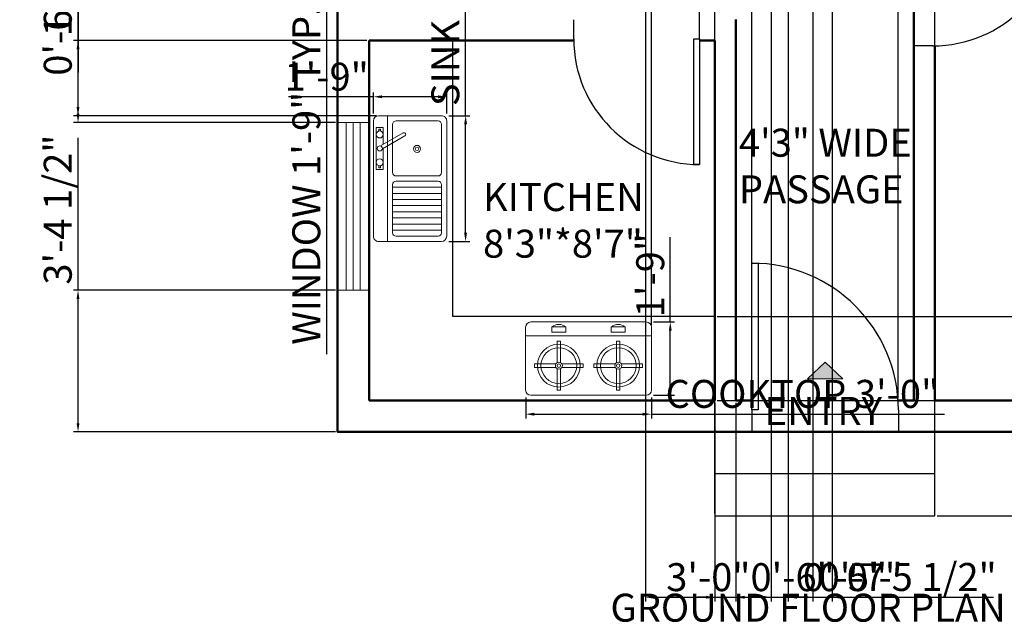
# Model space of a CAD drawing. Units: inches. Extents: x 2528 to 2954, y 1660 to 2209.
# Tile 1 of 4: x 2528 to 2810, y 1660 to 1832. Entities that reach past the tile are written whole.
import ezdxf

# ---------------------------------------------------------------- set-up
doc = ezdxf.new("R2010")
doc.units = ezdxf.units.IN
for name, color, linetype, lineweight in [('A-ANNO-DIMS', 5, 'Continuous', 18), ('A-ANNO-SYMB', 5, 'Continuous', 18), ('A-AREA-IDEN', 5, 'Continuous', 25), ('A-EQPM', 6, 'Continuous', 18), ('A-FLOR-CASE', 32, 'Continuous', 25), ('A-FLOR-FIXT', 6, 'Continuous', 18), ('DOOR', 3, 'Continuous', 25), ('STEPS', 30, 'Continuous', 25), ('TEXT', 5, 'Continuous', 25), ('WALL', 1, 'Continuous', 50), ('WINDOW', 4, 'Continuous', 18)]:
    doc.layers.add(name, color=color, linetype=linetype, lineweight=lineweight)
doc.styles.get("Standard").update_dxf_attribs({"font": 'arial.ttf'})
doc.dimstyles.new('ISO-25', dxfattribs={"dimtxt": 8, "dimasz": 2.5, "dimexe": 1.25, "dimexo": 0.625, "dimtad": 1, "dimlunit": 3, "dimtxsty": 'Standard', "dimcen": 2.5, "dimadec": 0, "dimazin": 0, "dimtfac": 1, "dimtmove": 0, "dimatfit": 3, "dimfxl": 1, "dimarcsym": 0})

# ---------------------------------------------------------------- blocks, each defined once
blk = doc.blocks.new('*U2')
for p, q in [((0, 0), (0, -6)), ((40, 0), (40, -6))]:
    blk.add_line(p, q)
blk.add_lwpolyline([(0, 0), (0, 40), (1.75, 40), (1.75, 0)], close=True)
blk.add_arc((0, 0), 40, 0, 90)
blk = doc.blocks.new('Faucet - kit sink top')
for p, q in [((-5.5, -0.75), (-5.5, -1.25)), ((-4.94278, -0.75), (-5.5, -0.75)), ((-5.5, -1.25), (-4.94278, -1.25)), ((-0.14775, -1.7441), (3.56698, -8.1782)), ((4.43301, -7.6782), (0.71828, -1.2441)), ((4.94278, -0.75), (5.5, -0.75)), ((5.5, -1.25), (4.94278, -1.25)), ((5.5, -0.75), (5.5, -1.25))]:
    blk.add_line(p, q)
blk.add_lwpolyline([(-0.00587, -2), (-6, -2), (-6, 0), (6, 0), (6, -2), (1.15195, -2)])
for centre, radius in [((-4, -1), 1), ((4, -1), 1), ((0, -1), 0.75)]:
    blk.add_circle(centre, radius)
blk.add_arc((4, -7.9282), 0.5, 210, 30)
blk = doc.blocks.new('sink')
for p, q in [((-18, -4), (18, -4)), ((-14.75, -19.5), (-14.75, -5.5)), ((-13, -19.5), (-13, -5.5)), ((-11.25, -19.5), (-11.25, -5.5)), ((-9.5, -19.5), (-9.5, -5.5)), ((-7.75, -19.5), (-7.75, -5.5)), ((-6, -19.5), (-6, -5.5)), ((-4.25, -19.5), (-4.25, -5.5)), ((-2.5, -19.5), (-2.5, -5.5)), ((-0.75, -18.5), (-0.75, -6.5)), ((0.75, -6.5), (0.75, -18.5))]:
    blk.add_line(p, q)
for points in [[(-16.5, 0), (16.5, 0)], [(-18, -19.5), (-18, -1.5)], [(18, -1.5), (18, -19.5)], [(-15.5, -5.5), (-1.75, -5.5)], [(1.75, -5.5), (15.5, -5.5)], [(-16.5, -18.5), (-16.5, -6.5)], [(16.5, -6.5), (16.5, -18.5)], [(-1.75, -19.5), (-15.5, -19.5)], [(15.5, -19.5), (1.75, -19.5)], [(16.5, -21), (-16.5, -21)]]:
    blk.add_lwpolyline(points)
for radius in [1, 0.5]:
    blk.add_circle((8.5, -12.5), radius)
for centre, radius, start, end in [((-16.5, -1.5), 1.5, 90, 180), ((16.5, -1.5), 1.5, 0, 90), ((-15.5, -6.5), 1, 90, 180), ((-1.75, -6.5), 1, 0, 90), ((1.75, -6.5), 1, 90, 180), ((15.5, -6.5), 1, 0, 90), ((-16.5, -19.5), 1.5, 180, 270), ((-15.5, -18.5), 1, 180, 270), ((-1.75, -18.5), 1, 270, 0), ((1.75, -18.5), 1, 180, 270), ((15.5, -18.5), 1, 270, 0), ((16.5, -19.5), 1.5, 270, 0)]:
    blk.add_arc(centre, radius, start, end)
blk.add_blockref('Faucet - kit sink top', (8.62, -0.83))
blk = doc.blocks.new('stove')
for p, q in [((2468.66, 1798.42), (2464.66, 1798.42)), ((2464.66, 1798.42), (2464.66, 1796.93)), ((2468.66, 1796.93), (2468.66, 1798.42)), ((2485.66, 1798.42), (2481.66, 1798.42)), ((2481.66, 1798.42), (2481.66, 1796.93)), ((2485.66, 1796.93), (2485.66, 1798.42)), ((2457.16, 1795.87), (2493.16, 1795.87)), ((2464.66, 1796.93), (2468.66, 1796.93)), ((2481.66, 1796.93), (2485.66, 1796.93))]:
    blk.add_line(p, q)
for points in [[(2457.16, 1780.37), (2457.16, 1798.37)], [(2458.66, 1799.87), (2491.66, 1799.87)], [(2493.16, 1798.37), (2493.16, 1780.37)], [(2491.66, 1778.87), (2458.66, 1778.87)]]:
    blk.add_lwpolyline(points)
for centre, radius in [((2466.66, 1787.37), 6.12), ((2483.66, 1787.37), 6.12), ((2466.66, 1787.37), 5.12), ((2483.66, 1787.37), 5.12), ((2466.66, 1787.37), 1), ((2466.66, 1787.37), 0.5), ((2483.66, 1787.37), 1), ((2483.66, 1787.37), 0.5)]:
    blk.add_circle(centre, radius)
for centre, radius, start, end in [((2458.66, 1798.37), 1.5, 90, 180), ((2466.66, 1796.04), 3.11, 49.9196, 130.0804), ((2483.66, 1796.04), 3.11, 49.9196, 130.0804), ((2491.66, 1798.37), 1.5, 0, 90), ((2458.66, 1780.37), 1.5, 180, 270), ((2491.66, 1780.37), 1.5, 270, 0)]:
    blk.add_arc(centre, radius, start, end)
blk = doc.blocks.new('stove kitchen')
for p, q in [((-9, 9.37), (-9, 15.48)), ((-9, 15.48), (-8, 15.48)), ((-8, 9.37), (-8, 15.48)), ((8, 9.37), (8, 15.48)), ((8, 15.48), (9, 15.48)), ((9, 9.37), (9, 15.48)), ((-9.37, 9), (-15.48, 9)), ((-15.48, 9), (-15.48, 8)), ((-7.63, 9), (-1.52, 9)), ((-1.52, 8), (-1.52, 9)), ((7.63, 9), (1.52, 9)), ((1.52, 9), (1.52, 8)), ((9.37, 9), (15.48, 9)), ((15.48, 8), (15.48, 9)), ((-9.37, 8), (-15.48, 8)), ((-9, 7.63), (-9, 1.52)), ((-8, 7.63), (-8, 1.52)), ((-7.63, 8), (-1.52, 8)), ((7.63, 8), (1.52, 8)), ((8, 7.63), (8, 1.52)), ((9, 7.63), (9, 1.52)), ((9.37, 8), (15.48, 8)), ((-8, 1.52), (-9, 1.52)), ((9, 1.52), (8, 1.52))]:
    blk.add_line(p, q)
blk.add_blockref('stove', (-2475.16, -1778.87))
blk = doc.blocks.new('WIN-48IN')
for p, q in [((0, 48), (9, 48)), ((2.5, 0), (2.5, 48)), ((4.5, 0), (4.5, 48)), ((6.5, 0), (6.5, 48)), ((9, 0), (0, 0))]:
    blk.add_line(p, q)
blk = doc.blocks.new('*D19')
at = {"layer": 'A-ANNO-DIMS', "color": 0, "lineweight": -2, "transparency": 16777216}
for p, q in [((2618.29, 1862.65), (2614.52, 1862.65)), ((2615.77, 1860.15), (2615.77, 1844.15)), ((2618.29, 1841.65), (2614.52, 1841.65)), ((2615.77, 1841.65), (2615.77, 1736.66))]:
    blk.add_line(p, q, dxfattribs=at)
at = {"layer": 'A-ANNO-DIMS', "color": 0, "transparency": 16777216}
for points in [[(2615.35, 1860.15), (2616.18, 1860.15), (2615.77, 1862.65)], [(2615.35, 1844.15), (2616.18, 1844.15), (2615.77, 1841.65)]]:
    blk.add_solid(points, dxfattribs=at)
at = {"layer": 'Defpoints', "color": 0, "transparency": 16777216}
for p in [(2618.92, 1862.65), (2615.77, 1841.65), (2618.92, 1841.65)]:
    blk.add_point(p, dxfattribs=at)
at = {"layer": 'A-ANNO-DIMS', "color": 0, "transparency": 16777216, "insert": (2611, 1787.9), "char_height": 8, "attachment_point": 5, "rotation": 90}
blk.add_mtext('WINDOW 1\'-9" TYP.', dxfattribs=at)
blk = doc.blocks.new('*D23')
at = {"layer": 'A-ANNO-DIMS', "color": 0, "lineweight": -2, "transparency": 16777216}
for p, q in [((2655.56, 1804.89), (2655.56, 1859.06)), ((2650.79, 1804.89), (2656.81, 1804.89)), ((2655.56, 1771.39), (2655.56, 1802.39)), ((2650.79, 1768.89), (2656.81, 1768.89))]:
    blk.add_line(p, q, dxfattribs=at)
at = {"layer": 'A-ANNO-DIMS', "color": 0, "transparency": 16777216}
for points in [[(2655.15, 1802.39), (2655.98, 1802.39), (2655.56, 1804.89)], [(2655.15, 1771.39), (2655.98, 1771.39), (2655.56, 1768.89)]]:
    blk.add_solid(points, dxfattribs=at)
at = {"layer": 'Defpoints', "color": 0, "transparency": 16777216}
for p in [(2650.16, 1804.89), (2655.56, 1804.89), (2650.16, 1768.89)]:
    blk.add_point(p, dxfattribs=at)
at = {"layer": 'A-ANNO-DIMS', "color": 0, "transparency": 16777216, "insert": (2650.8, 1833.22), "char_height": 8, "attachment_point": 5, "rotation": 90}
blk.add_mtext('SINK 3\'-0"', dxfattribs=at)
blk = doc.blocks.new('*D24')
at = {"layer": 'A-ANNO-DIMS', "color": 0, "lineweight": -2, "transparency": 16777216}
for p, q in [((2629.16, 1810.29), (2604.9, 1810.29)), ((2629.16, 1805.51), (2629.16, 1811.54)), ((2647.66, 1810.29), (2631.66, 1810.29)), ((2650.16, 1805.51), (2650.16, 1811.54))]:
    blk.add_line(p, q, dxfattribs=at)
at = {"layer": 'A-ANNO-DIMS', "color": 0, "transparency": 16777216}
for points in [[(2631.66, 1810.71), (2631.66, 1809.87), (2629.16, 1810.29)], [(2647.66, 1810.71), (2647.66, 1809.87), (2650.16, 1810.29)]]:
    blk.add_solid(points, dxfattribs=at)
at = {"layer": 'Defpoints', "color": 0, "transparency": 16777216}
for p in [(2629.16, 1810.29), (2629.16, 1804.89), (2650.16, 1804.89)]:
    blk.add_point(p, dxfattribs=at)
at = {"layer": 'A-ANNO-DIMS', "color": 0, "transparency": 16777216, "insert": (2615.78, 1815), "char_height": 8, "attachment_point": 5}
blk.add_mtext('1\'-9"', dxfattribs=at)
blk = doc.blocks.new('*D25')
at = {"layer": 'A-ANNO-DIMS', "color": 0, "lineweight": -2, "transparency": 16777216}
for p, q in [((2672.76, 1724.24), (2672.76, 1718.22)), ((2708.76, 1724.24), (2708.76, 1718.22)), ((2675.26, 1719.47), (2706.26, 1719.47)), ((2708.76, 1719.47), (2792.67, 1719.47))]:
    blk.add_line(p, q, dxfattribs=at)
at = {"layer": 'A-ANNO-DIMS', "color": 0, "transparency": 16777216}
for points in [[(2675.26, 1719.89), (2675.26, 1719.05), (2672.76, 1719.47)], [(2706.26, 1719.89), (2706.26, 1719.05), (2708.76, 1719.47)]]:
    blk.add_solid(points, dxfattribs=at)
at = {"layer": 'Defpoints', "color": 0, "transparency": 16777216}
for p in [(2672.76, 1724.87), (2708.76, 1724.87), (2708.76, 1719.47)]:
    blk.add_point(p, dxfattribs=at)
at = {"layer": 'A-ANNO-DIMS', "color": 0, "transparency": 16777216, "insert": (2751.96, 1724.24), "char_height": 8, "attachment_point": 5}
blk.add_mtext('COOKTOP 3\'-0"', dxfattribs=at)
blk = doc.blocks.new('*D26')
at = {"layer": 'A-ANNO-DIMS', "color": 0, "lineweight": -2, "transparency": 16777216}
for p, q in [((2714.16, 1745.87), (2714.16, 1770.13)), ((2709.38, 1745.87), (2715.41, 1745.87)), ((2714.16, 1727.37), (2714.16, 1743.37)), ((2709.38, 1724.87), (2715.41, 1724.87))]:
    blk.add_line(p, q, dxfattribs=at)
at = {"layer": 'A-ANNO-DIMS', "color": 0, "transparency": 16777216}
for points in [[(2713.74, 1743.37), (2714.57, 1743.37), (2714.16, 1745.87)], [(2713.74, 1727.37), (2714.57, 1727.37), (2714.16, 1724.87)]]:
    blk.add_solid(points, dxfattribs=at)
at = {"layer": 'Defpoints', "color": 0, "transparency": 16777216}
for p in [(2708.76, 1745.87), (2714.16, 1745.87), (2708.76, 1724.87)]:
    blk.add_point(p, dxfattribs=at)
at = {"layer": 'A-ANNO-DIMS', "color": 0, "transparency": 16777216, "insert": (2709.45, 1759.25), "char_height": 8, "attachment_point": 5, "rotation": 90}
blk.add_mtext('1\'-9"', dxfattribs=at)
blk = doc.blocks.new('*D27')
at = {"layer": 'A-ANNO-DIMS', "color": 0, "lineweight": -2, "transparency": 16777216}
for p, q in [((2544.62, 1754.93), (2544.62, 1798.58)), ((2618.29, 1754.93), (2543.37, 1754.93)), ((2544.62, 1716.89), (2544.62, 1752.43)), ((2618.29, 1714.39), (2543.37, 1714.39))]:
    blk.add_line(p, q, dxfattribs=at)
at = {"layer": 'A-ANNO-DIMS', "color": 0, "transparency": 16777216}
for points in [[(2544.2, 1752.43), (2545.03, 1752.43), (2544.62, 1754.93)], [(2544.2, 1716.89), (2545.03, 1716.89), (2544.62, 1714.39)]]:
    blk.add_solid(points, dxfattribs=at)
at = {"layer": 'Defpoints', "color": 0, "transparency": 16777216}
for p in [(2544.62, 1754.93), (2618.92, 1754.93), (2618.92, 1714.39)]:
    blk.add_point(p, dxfattribs=at)
at = {"layer": 'A-ANNO-DIMS', "color": 0, "transparency": 16777216, "insert": (2539.85, 1778), "char_height": 8, "attachment_point": 5, "rotation": 90}
blk.add_mtext('3\'-4 1/2"', dxfattribs=at)
blk = doc.blocks.new('*D28')
at = {"layer": 'A-ANNO-DIMS', "color": 0, "lineweight": -2, "transparency": 16777216}
for p, q in [((2544.62, 1841.65), (2544.62, 1885.3)), ((2618.29, 1841.65), (2543.37, 1841.65)), ((2544.62, 1805.43), (2544.62, 1839.14)), ((2618.29, 1802.93), (2543.37, 1802.93))]:
    blk.add_line(p, q, dxfattribs=at)
at = {"layer": 'A-ANNO-DIMS', "color": 0, "transparency": 16777216}
for points in [[(2544.2, 1839.14), (2545.03, 1839.14), (2544.62, 1841.65)], [(2544.2, 1805.43), (2545.03, 1805.43), (2544.62, 1802.93)]]:
    blk.add_solid(points, dxfattribs=at)
at = {"layer": 'Defpoints', "color": 0, "transparency": 16777216}
for p in [(2544.62, 1841.65), (2618.92, 1841.65), (2618.92, 1802.93)]:
    blk.add_point(p, dxfattribs=at)
at = {"layer": 'A-ANNO-DIMS', "color": 0, "transparency": 16777216, "insert": (2539.85, 1864.72), "char_height": 8, "attachment_point": 5, "rotation": 90}
blk.add_mtext('3\'-2 1/2"', dxfattribs=at)
blk = doc.blocks.new('*D34')
at = {"layer": 'A-ANNO-DIMS', "color": 0, "lineweight": -2, "transparency": 16777216}
for p, q in [((2618.92, 1715.01), (2618.92, 2122.94)), ((2726.92, 1703.01), (2726.92, 2122.94)), ((2621.42, 2121.69), (2724.42, 2121.69))]:
    blk.add_line(p, q, dxfattribs=at)
at = {"layer": 'A-ANNO-DIMS', "color": 0, "transparency": 16777216}
for points in [[(2621.42, 2122.11), (2621.42, 2121.27), (2618.92, 2121.69)], [(2724.42, 2122.11), (2724.42, 2121.27), (2726.92, 2121.69)]]:
    blk.add_solid(points, dxfattribs=at)
at = {"layer": 'Defpoints', "color": 0, "transparency": 16777216}
for p in [(2726.92, 2121.69), (2618.92, 1714.39), (2726.92, 1702.39)]:
    blk.add_point(p, dxfattribs=at)
at = {"layer": 'A-ANNO-DIMS', "color": 0, "transparency": 16777216, "insert": (2672.92, 2126.4), "char_height": 8, "attachment_point": 5}
blk.add_mtext('9\'-0"', dxfattribs=at)
blk = doc.blocks.new('*D35')
at = {"layer": 'A-ANNO-DIMS', "color": 0, "lineweight": -2, "transparency": 16777216}
for p, q in [((2726.92, 1691.01), (2726.92, 2122.94)), ((2789.92, 1691.01), (2789.92, 2122.94)), ((2729.42, 2121.69), (2787.42, 2121.69))]:
    blk.add_line(p, q, dxfattribs=at)
at = {"layer": 'A-ANNO-DIMS', "color": 0, "transparency": 16777216}
for points in [[(2729.42, 2122.11), (2729.42, 2121.27), (2726.92, 2121.69)], [(2787.42, 2122.11), (2787.42, 2121.27), (2789.92, 2121.69)]]:
    blk.add_solid(points, dxfattribs=at)
at = {"layer": 'Defpoints', "color": 0, "transparency": 16777216}
for p in [(2789.92, 2121.69), (2726.92, 1690.39), (2789.92, 1690.39)]:
    blk.add_point(p, dxfattribs=at)
at = {"layer": 'A-ANNO-DIMS', "color": 0, "transparency": 16777216, "insert": (2758.42, 2126.4), "char_height": 8, "attachment_point": 5}
blk.add_mtext('5\'-3"', dxfattribs=at)
blk = doc.blocks.new('*D36')
at = {"layer": 'A-ANNO-DIMS', "color": 0, "lineweight": -2, "transparency": 16777216}
for p, q in [((2790.54, 1714.39), (2943.47, 1714.39)), ((2942.22, 1692.89), (2942.22, 1711.89)), ((2790.54, 1690.39), (2943.47, 1690.39))]:
    blk.add_line(p, q, dxfattribs=at)
at = {"layer": 'A-ANNO-DIMS', "color": 0, "transparency": 16777216}
for points in [[(2941.8, 1711.89), (2942.63, 1711.89), (2942.22, 1714.39)], [(2941.8, 1692.89), (2942.63, 1692.89), (2942.22, 1690.39)]]:
    blk.add_solid(points, dxfattribs=at)
at = {"layer": 'Defpoints', "color": 0, "transparency": 16777216}
for p in [(2789.92, 1714.39), (2942.22, 1714.39), (2789.92, 1690.39)]:
    blk.add_point(p, dxfattribs=at)
at = {"layer": 'A-ANNO-DIMS', "color": 0, "transparency": 16777216, "insert": (2937.51, 1702.39), "char_height": 8, "attachment_point": 5, "rotation": 90}
blk.add_mtext('2\'-0"', dxfattribs=at)
blk = doc.blocks.new('*D37')
at = {"layer": 'A-ANNO-DIMS', "color": 0, "lineweight": -2, "transparency": 16777216}
for p, q in [((2737.46, 1724.01), (2737.46, 2122.94)), ((2779.37, 1724.01), (2779.37, 2122.94)), ((2739.96, 2121.69), (2776.87, 2121.69))]:
    blk.add_line(p, q, dxfattribs=at)
at = {"layer": 'A-ANNO-DIMS', "color": 0, "transparency": 16777216}
for points in [[(2739.96, 2122.11), (2739.96, 2121.27), (2737.46, 2121.69)], [(2776.87, 2122.11), (2776.87, 2121.27), (2779.37, 2121.69)]]:
    blk.add_solid(points, dxfattribs=at)
at = {"layer": 'Defpoints', "color": 0, "transparency": 16777216}
for p in [(2779.37, 2121.69), (2737.46, 1723.39), (2779.37, 1723.39)]:
    blk.add_point(p, dxfattribs=at)
at = {"layer": 'A-ANNO-DIMS', "color": 0, "transparency": 16777216, "insert": (2758.42, 2126.4), "char_height": 8, "attachment_point": 5}
blk.add_mtext('3\'-6"', dxfattribs=at)
blk = doc.blocks.new('*D38')
at = {"layer": 'A-ANNO-DIMS', "color": 0, "lineweight": -2, "transparency": 16777216}
for p, q in [((2707.05, 1956.76), (2707.05, 1665.84)), ((2743.05, 1956.76), (2743.05, 1665.84)), ((2709.55, 1667.09), (2740.55, 1667.09))]:
    blk.add_line(p, q, dxfattribs=at)
at = {"layer": 'A-ANNO-DIMS', "color": 0, "transparency": 16777216}
for points in [[(2709.55, 1667.51), (2709.55, 1666.67), (2707.05, 1667.09)], [(2740.55, 1667.51), (2740.55, 1666.67), (2743.05, 1667.09)]]:
    blk.add_solid(points, dxfattribs=at)
at = {"layer": 'Defpoints', "color": 0, "transparency": 16777216}
for p in [(2707.05, 1957.39), (2743.05, 1957.39), (2743.05, 1667.09)]:
    blk.add_point(p, dxfattribs=at)
at = {"layer": 'A-ANNO-DIMS', "color": 0, "transparency": 16777216, "insert": (2725.05, 1671.8), "char_height": 8, "attachment_point": 5}
blk.add_mtext('3\'-0"', dxfattribs=at)
blk = doc.blocks.new('*D44')
at = {"layer": 'A-ANNO-DIMS', "color": 0, "lineweight": -2, "transparency": 16777216}
for p, q in [((2727.54, 1747.39), (2943.47, 1747.39)), ((2942.22, 1725.89), (2942.22, 1744.89)), ((2727.54, 1723.39), (2943.47, 1723.39))]:
    blk.add_line(p, q, dxfattribs=at)
at = {"layer": 'A-ANNO-DIMS', "color": 0, "transparency": 16777216}
for points in [[(2941.8, 1744.89), (2942.63, 1744.89), (2942.22, 1747.39)], [(2941.8, 1725.89), (2942.63, 1725.89), (2942.22, 1723.39)]]:
    blk.add_solid(points, dxfattribs=at)
at = {"layer": 'Defpoints', "color": 0, "transparency": 16777216}
for p in [(2726.92, 1747.39), (2942.22, 1747.39), (2726.92, 1723.39)]:
    blk.add_point(p, dxfattribs=at)
at = {"layer": 'A-ANNO-DIMS', "color": 0, "transparency": 16777216, "insert": (2937.51, 1735.39), "char_height": 8, "attachment_point": 5, "rotation": 90}
blk.add_mtext('2\'-0"', dxfattribs=at)
blk = doc.blocks.new('*D45')
at = {"layer": 'A-ANNO-DIMS', "color": 0, "lineweight": -2, "transparency": 16777216}
for p, q in [((2708.76, 1744.99), (2708.76, 2122.94)), ((2726.92, 1748.01), (2726.92, 2122.94)), ((2711.26, 2121.69), (2724.42, 2121.69)), ((2726.92, 2121.69), (2751.18, 2121.69))]:
    blk.add_line(p, q, dxfattribs=at)
at = {"layer": 'A-ANNO-DIMS', "color": 0, "transparency": 16777216}
for points in [[(2711.26, 2122.11), (2711.26, 2121.27), (2708.76, 2121.69)], [(2724.42, 2122.11), (2724.42, 2121.27), (2726.92, 2121.69)]]:
    blk.add_solid(points, dxfattribs=at)
at = {"layer": 'Defpoints', "color": 0, "transparency": 16777216}
for p in [(2726.92, 2121.69), (2726.92, 1747.39), (2708.76, 1744.37)]:
    blk.add_point(p, dxfattribs=at)
at = {"layer": 'A-ANNO-DIMS', "color": 0, "transparency": 16777216, "insert": (2740.3, 2126.4), "char_height": 8, "attachment_point": 5}
blk.add_mtext('1\'-6"', dxfattribs=at)
blk = doc.blocks.new('*D46')
at = {"layer": 'A-ANNO-DIMS', "color": 0, "lineweight": -2, "transparency": 16777216}
for p, q in [((2544.62, 1826.39), (2544.62, 1869.29)), ((2627.29, 1826.39), (2543.37, 1826.39)), ((2544.62, 1807.39), (2544.62, 1823.89)), ((2630.04, 1804.89), (2543.37, 1804.89))]:
    blk.add_line(p, q, dxfattribs=at)
at = {"layer": 'A-ANNO-DIMS', "color": 0, "transparency": 16777216}
for points in [[(2544.2, 1823.89), (2545.03, 1823.89), (2544.62, 1826.39)], [(2544.2, 1807.39), (2545.03, 1807.39), (2544.62, 1804.89)]]:
    blk.add_solid(points, dxfattribs=at)
at = {"layer": 'Defpoints', "color": 0, "transparency": 16777216}
for p in [(2544.62, 1826.39), (2627.92, 1826.39), (2630.66, 1804.89)]:
    blk.add_point(p, dxfattribs=at)
at = {"layer": 'A-ANNO-DIMS', "color": 0, "transparency": 16777216, "insert": (2539.85, 1849.09), "char_height": 8, "attachment_point": 5, "rotation": 90}
blk.add_mtext('1\'-9 1/2"', dxfattribs=at)
blk = doc.blocks.new('*D48')
at = {"layer": 'A-ANNO-DIMS', "color": 0, "lineweight": -2, "transparency": 16777216}
for p, q in [((2747.92, 2088.76), (2747.92, 1665.84)), ((2754.92, 2088.76), (2754.92, 1665.84)), ((2750.42, 1667.09), (2752.42, 1667.09)), ((2754.92, 1667.09), (2779.93, 1667.09))]:
    blk.add_line(p, q, dxfattribs=at)
at = {"layer": 'A-ANNO-DIMS', "color": 0, "transparency": 16777216}
for points in [[(2750.42, 1667.51), (2750.42, 1666.67), (2747.92, 1667.09)], [(2752.42, 1667.51), (2752.42, 1666.67), (2754.92, 1667.09)]]:
    blk.add_solid(points, dxfattribs=at)
at = {"layer": 'Defpoints', "color": 0, "transparency": 16777216}
for p in [(2747.92, 2089.39), (2754.92, 2089.39), (2754.92, 1667.09)]:
    blk.add_point(p, dxfattribs=at)
at = {"layer": 'A-ANNO-DIMS', "color": 0, "transparency": 16777216, "insert": (2768.67, 1671.8), "char_height": 8, "attachment_point": 5}
blk.add_mtext('0\'-7"', dxfattribs=at)
blk = doc.blocks.new('*D49')
at = {"layer": 'A-ANNO-DIMS', "color": 0, "lineweight": -2, "transparency": 16777216}
for p, q in [((2747.92, 1956.76), (2747.92, 1665.84)), ((2743.05, 1950.76), (2743.05, 1665.84)), ((2740.55, 1667.09), (2738.05, 1667.09)), ((2743.05, 1667.09), (2747.92, 1667.09)), ((2750.42, 1667.09), (2775.43, 1667.09))]:
    blk.add_line(p, q, dxfattribs=at)
at = {"layer": 'A-ANNO-DIMS', "color": 0, "transparency": 16777216}
for points in [[(2740.55, 1667.51), (2740.55, 1666.67), (2743.05, 1667.09)], [(2750.42, 1667.51), (2750.42, 1666.67), (2747.92, 1667.09)]]:
    blk.add_solid(points, dxfattribs=at)
at = {"layer": 'Defpoints', "color": 0, "transparency": 16777216}
for p in [(2747.92, 1957.39), (2743.05, 1951.39), (2747.92, 1667.09)]:
    blk.add_point(p, dxfattribs=at)
at = {"layer": 'A-ANNO-DIMS', "color": 0, "transparency": 16777216, "insert": (2764.17, 1671.8), "char_height": 8, "attachment_point": 5}
blk.add_mtext('0\'-5"', dxfattribs=at)
blk = doc.blocks.new('*D50')
at = {"layer": 'A-ANNO-DIMS', "color": 0, "lineweight": -2, "transparency": 16777216}
for p, q in [((2754.92, 1956.76), (2754.92, 1665.84)), ((2760.54, 1950.76), (2760.54, 1665.84)), ((2752.42, 1667.09), (2749.92, 1667.09)), ((2754.92, 1667.09), (2760.54, 1667.09)), ((2763.04, 1667.09), (2806.7, 1667.09))]:
    blk.add_line(p, q, dxfattribs=at)
at = {"layer": 'A-ANNO-DIMS', "color": 0, "transparency": 16777216}
for points in [[(2752.42, 1667.51), (2752.42, 1666.67), (2754.92, 1667.09)], [(2763.04, 1667.51), (2763.04, 1666.67), (2760.54, 1667.09)]]:
    blk.add_solid(points, dxfattribs=at)
at = {"layer": 'Defpoints', "color": 0, "transparency": 16777216}
for p in [(2754.92, 1957.39), (2760.54, 1951.39), (2760.54, 1667.09)]:
    blk.add_point(p, dxfattribs=at)
at = {"layer": 'A-ANNO-DIMS', "color": 0, "transparency": 16777216, "insert": (2786.12, 1671.85), "char_height": 8, "attachment_point": 5}
blk.add_mtext('0\'-5 1/2"', dxfattribs=at)
blk = doc.blocks.new('*D51')
at = {"layer": 'A-ANNO-DIMS', "color": 0, "lineweight": -2, "transparency": 16777216}
for p, q in [((2789.29, 1867.39), (2543.37, 1867.39)), ((2544.62, 1864.89), (2544.62, 1863.37)), ((2783.29, 1860.87), (2543.37, 1860.87)), ((2544.62, 1860.87), (2544.62, 1817.21))]:
    blk.add_line(p, q, dxfattribs=at)
at = {"layer": 'A-ANNO-DIMS', "color": 0, "transparency": 16777216}
for points in [[(2544.2, 1864.89), (2545.03, 1864.89), (2544.62, 1867.39)], [(2544.2, 1863.37), (2545.03, 1863.37), (2544.62, 1860.87)]]:
    blk.add_solid(points, dxfattribs=at)
at = {"layer": 'Defpoints', "color": 0, "transparency": 16777216}
for p in [(2789.92, 1867.39), (2544.62, 1860.87), (2783.92, 1860.87)]:
    blk.add_point(p, dxfattribs=at)
at = {"layer": 'A-ANNO-DIMS', "color": 0, "transparency": 16777216, "insert": (2539.85, 1837.79), "char_height": 8, "attachment_point": 5, "rotation": 90}
blk.add_mtext('0\'-6 1/2"', dxfattribs=at)
blk = doc.blocks.new('*D54')
at = {"layer": 'A-ANNO-DIMS', "color": 0, "lineweight": -2, "transparency": 16777216}
for p, q in [((2722.51, 1827.01), (2722.51, 2122.94)), ((2726.92, 1827.01), (2726.92, 2122.94)), ((2720.01, 2121.69), (2717.51, 2121.69)), ((2722.51, 2121.69), (2726.92, 2121.69)), ((2729.42, 2121.69), (2773.07, 2121.69))]:
    blk.add_line(p, q, dxfattribs=at)
at = {"layer": 'A-ANNO-DIMS', "color": 0, "transparency": 16777216}
for points in [[(2720.01, 2122.11), (2720.01, 2121.27), (2722.51, 2121.69)], [(2729.42, 2122.11), (2729.42, 2121.27), (2726.92, 2121.69)]]:
    blk.add_solid(points, dxfattribs=at)
at = {"layer": 'Defpoints', "color": 0, "transparency": 16777216}
for p in [(2726.92, 2121.69), (2722.51, 1826.39), (2726.92, 1826.39)]:
    blk.add_point(p, dxfattribs=at)
at = {"layer": 'A-ANNO-DIMS', "color": 0, "transparency": 16777216, "insert": (2752.49, 2126.45), "char_height": 8, "attachment_point": 5}
blk.add_mtext('0\'-4 1/2"', dxfattribs=at)
blk = doc.blocks.new('*D55')
at = {"layer": 'A-ANNO-DIMS', "color": 0, "lineweight": -2, "transparency": 16777216}
for p, q in [((2726.92, 1722.76), (2726.92, 1665.84)), ((2732.92, 1722.76), (2732.92, 1665.84)), ((2724.42, 1667.09), (2721.92, 1667.09)), ((2726.92, 1667.09), (2732.92, 1667.09)), ((2735.42, 1667.09), (2760.43, 1667.09))]:
    blk.add_line(p, q, dxfattribs=at)
at = {"layer": 'A-ANNO-DIMS', "color": 0, "transparency": 16777216}
for points in [[(2724.42, 1667.51), (2724.42, 1666.67), (2726.92, 1667.09)], [(2735.42, 1667.51), (2735.42, 1666.67), (2732.92, 1667.09)]]:
    blk.add_solid(points, dxfattribs=at)
at = {"layer": 'Defpoints', "color": 0, "transparency": 16777216}
for p in [(2726.92, 1723.39), (2732.92, 1723.39), (2732.92, 1667.09)]:
    blk.add_point(p, dxfattribs=at)
at = {"layer": 'A-ANNO-DIMS', "color": 0, "transparency": 16777216, "insert": (2749.17, 1671.8), "char_height": 8, "attachment_point": 5}
blk.add_mtext('0\'-6"', dxfattribs=at)

msp = doc.modelspace()

# ---------------------------------------------------------------- hatches: boundary and pattern name
at = {"layer": 'A-ANNO-SYMB'}
h = msp.add_hatch(color=256, dxfattribs=at)
h.dxf.hatch_style = 1
h.paths.add_polyline_path([(2758.527, 1734.365), (2753.476, 1729.547), (2763.578, 1729.547)])

# ---------------------------------------------------------------- linework, layer by layer
for p, q in [((2753.476, 1729.547), (2758.527, 1734.365)), ((2763.578, 1729.547), (2758.527, 1734.365)), ((2753.476, 1729.547), (2763.578, 1729.547))]:
    msp.add_line(p, q, dxfattribs=at)
at = {"layer": 'A-FLOR-CASE'}
for p, q in [((2651.915, 1747.389), (2651.915, 1826.389)), ((2726.915, 1747.389), (2651.915, 1747.389))]:
    msp.add_line(p, q, dxfattribs=at)
at = {"layer": 'STEPS'}
for p, q in [((2726.915, 1714.389), (2726.915, 1690.389)), ((2789.915, 1690.389), (2789.915, 1714.389)), ((2789.915, 1702.389), (2726.915, 1702.389)), ((2726.915, 1690.389), (2789.915, 1690.389))]:
    msp.add_line(p, q, dxfattribs=at)
at = {"layer": 'WALL'}
for p, q in [((2783.915, 1873.389), (2783.915, 1723.389)), ((2732.915, 1723.389), (2732.915, 1832.389)), ((2627.915, 1723.389), (2627.915, 1826.389)), ((2686.511, 1826.389), (2627.915, 1826.389)), ((2726.915, 1826.389), (2722.508, 1826.389)), ((2726.915, 1723.389), (2726.915, 1826.389)), ((2789.915, 1824.871), (2789.915, 1723.389)), ((2726.915, 1723.389), (2627.915, 1723.389)), ((2737.461, 1723.389), (2732.915, 1723.389)), ((2783.915, 1723.389), (2779.374, 1723.389)), ((2909.915, 1723.389), (2789.915, 1723.389))]:
    msp.add_line(p, q, dxfattribs=at)
msp.add_lwpolyline([(2618.915, 2098.389), (2918.915, 2098.389), (2918.915, 1714.389), (2618.915, 1714.389)], close=True, dxfattribs=at)

# ---------------------------------------------------------------- block references
at = {"layer": 'A-EQPM'}
msp.add_blockref('stove kitchen', (2690.757, 1724.869), dxfattribs=at)
at = {"layer": 'A-FLOR-FIXT', "rotation": 89.99999999999999}
msp.add_blockref('sink', (2629.165, 1786.889), dxfattribs=at)
at = {"layer": 'DOOR', "xscale": 0.9, "yscale": 0.9, "zscale": 0.9}
for p, rotation in [((2789.315, 1860.866), 270), ((2722.508, 1826.912), 180)]:
    msp.add_blockref('*U2', p, dxfattribs=dict(at, rotation=rotation))
at = {"layer": 'DOOR', "xscale": 1.05, "yscale": 1.05, "zscale": 1.05}
msp.add_blockref('*U2', (2737.461, 1720.689), dxfattribs=at)
at = {"layer": 'WINDOW', "rotation": 180}
msp.add_blockref('WIN-48IN', (2627.915, 1802.925), dxfattribs=at)

# ---------------------------------------------------------------- texts
at = {"layer": 'A-AREA-IDEN', "char_height": 8, "attachment_point": 1}
for s, width, insert in [('4\'3" WIDE\\PPASSAGE', 170.32858, (2733.802, 1801.148)), ('KITCHEN\\P8\'3"*8\'7"', 15.41436, (2660.56, 1785.593))]:
    msp.add_mtext_dynamic_manual_height_columns(s, width=width, gutter_width=12.5, heights=[0], dxfattribs=dict(at, insert=insert))
at = {"layer": 'TEXT', "char_height": 8, "attachment_point": 1}
for s, width, insert in [('ENTRY', 22.49042, (2741.157, 1724.404)), ('GROUND FLOOR PLAN', 158.72813, (2697.024, 1668.1))]:
    msp.add_mtext_dynamic_manual_height_columns(s, width=width, gutter_width=12.5, heights=[0], dxfattribs=dict(at, insert=insert))

# ---------------------------------------------------------------- dimensions: what is measured, and where the dimension line sits
at = {"layer": 'A-ANNO-DIMS'}
for base, p1, p2, picture, middle in [((2726.915, 2121.689), (2722.508, 1826.389), (2726.915, 1826.389), '*D54', (2752.494, 2126.451)), ((2726.915, 2121.689), (2618.915, 1714.389), (2726.915, 1702.389), '*D34', (2672.915, 2126.399)), ((2726.915, 2121.689), (2708.757, 1744.369), (2726.915, 1747.389), '*D45', (2740.296, 2126.399)), ((2789.915, 2121.689), (2726.915, 1690.389), (2789.915, 1690.389), '*D35', (2758.415, 2126.402)), ((2779.374, 2121.689), (2737.461, 1723.389), (2779.374, 1723.389), '*D37', (2758.418, 2126.402)), ((2754.915, 1667.089), (2747.915, 2089.389), (2754.915, 2089.389), '*D48', (2768.673, 1671.799)), ((2743.048, 1667.089), (2707.053, 1957.389), (2743.048, 1957.389), '*D38', (2725.051, 1671.802)), ((2747.915, 1667.089), (2743.048, 1951.389), (2747.915, 1957.389), '*D49', (2764.173, 1671.799)), ((2760.539, 1667.089), (2754.915, 1957.389), (2760.539, 1951.389), '*D50', (2786.117, 1671.851)), ((2732.915, 1667.089), (2726.915, 1723.389), (2732.915, 1723.389), '*D55', (2749.173, 1671.799))]:
    dim = msp.add_linear_dim(base=base, p1=p1, p2=p2, dimstyle='ISO-25', override={"dimdec": 1, "dimlfac": 1, "dimrnd": 0, "dimzin": 1, "dimdsep": 46, "dimlunit": 4, "dimfrac": 2}, dxfattribs=at)
    dim.commit()
    dim.dimension.update_dxf_attribs({"geometry": picture, "text_midpoint": middle})
for base, p1, p2, angle, picture, middle in [((2544.615, 1841.645), (2618.915, 1802.925), (2618.915, 1841.645), 90, '*D28', (2539.851, 1864.721)), ((2544.615, 1826.389), (2630.665, 1804.889), (2627.915, 1826.389), 90, '*D46', (2539.854, 1849.091)), ((2544.615, 1860.866), (2789.915, 1867.389), (2783.915, 1860.866), 90, '*D51', (2539.854, 1837.787)), ((2629.165, 1810.289), (2650.165, 1804.889), (2629.165, 1804.889), 180, '*D24', (2615.784, 1814.999)), ((2544.615, 1754.925), (2618.915, 1714.389), (2618.915, 1754.925), 90, '*D27', (2539.851, 1778.001)), ((2714.157, 1745.869), (2708.757, 1724.869), (2708.757, 1745.869), 90, '*D26', (2709.447, 1759.25)), ((2942.215, 1747.389), (2726.915, 1723.389), (2726.915, 1747.389), 90, '*D44', (2937.505, 1735.389)), ((2942.215, 1714.389), (2789.915, 1690.389), (2789.915, 1714.389), 90, '*D36', (2937.505, 1702.389))]:
    dim = msp.add_linear_dim(base=base, p1=p1, p2=p2, angle=angle, dimstyle='ISO-25', override={"dimdec": 1, "dimlfac": 1, "dimrnd": 0, "dimzin": 1, "dimdsep": 46, "dimlunit": 4, "dimfrac": 2}, dxfattribs=at)
    dim.commit()
    dim.dimension.update_dxf_attribs({"geometry": picture, "text_midpoint": middle})
for base, p1, p2, angle, text, picture, middle in [((2615.765, 1841.645), (2618.915, 1862.645), (2618.915, 1841.645), 270, 'WINDOW <> TYP.', '*D19', (2611.001, 1787.903)), ((2655.565, 1804.889), (2650.165, 1768.889), (2650.165, 1804.889), 90, 'SINK <>', '*D23', (2650.801, 1833.223))]:
    dim = msp.add_linear_dim(base=base, p1=p1, p2=p2, angle=angle, text=text, dimstyle='ISO-25', override={"dimdec": 1, "dimlfac": 1, "dimrnd": 0, "dimzin": 1, "dimdsep": 46, "dimlunit": 4, "dimfrac": 2}, dxfattribs=at)
    dim.commit()
    dim.dimension.update_dxf_attribs({"geometry": picture, "text_midpoint": middle})
dim = msp.add_linear_dim(base=(2708.757, 1719.469), p1=(2672.757, 1724.869), p2=(2708.757, 1724.869), text='COOKTOP <>', dimstyle='ISO-25', override={"dimdec": 1, "dimlfac": 1, "dimrnd": 0, "dimzin": 1, "dimdsep": 46, "dimlunit": 4, "dimfrac": 2}, dxfattribs=at)
dim.commit()
dim.dimension.update_dxf_attribs({"geometry": '*D25', "text_midpoint": (2751.964, 1724.236)})

doc.saveas('drawing.dxf')
